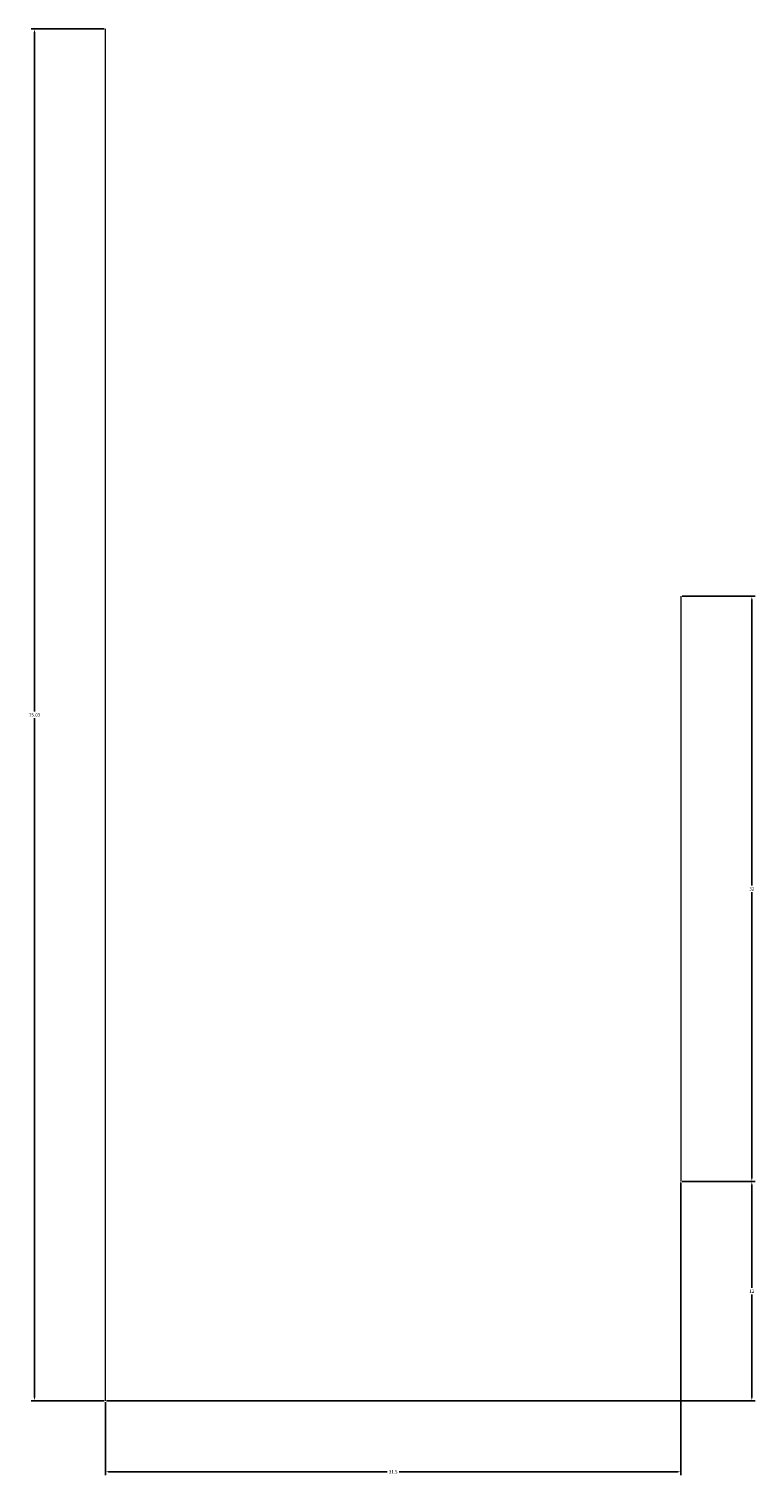
# Model space of a CAD drawing. Units: millimetres. Extents: x 554.6 to 594.4, y 996.2 to 1075.2.
import ezdxf

# ---------------------------------------------------------------- set-up
doc = ezdxf.new("R2010")
doc.units = ezdxf.units.MM
doc.layers.add('M-CONS', color=7, linetype='Continuous', lineweight=13)
doc.layers.add('M-DIMS', color=2, linetype='Continuous', lineweight=18)
doc.styles.get("Standard").update_dxf_attribs({"font": 'arial.ttf'})
doc.dimstyles.get("Standard").update_dxf_attribs({"dimtxt": 0.18, "dimasz": 0.18, "dimexe": 0.18, "dimexo": 0.0625, "dimgap": 0.09, "dimtad": 0, "dimtih": 1, "dimtoh": 1, "dimdec": 4, "dimzin": 0, "dimdsep": 46, "dimtxsty": 'Standard', "dimcen": 0.09, "dimadec": 0, "dimazin": 0, "dimtfac": 1, "dimtdec": 4, "dimtofl": 0, "dimtmove": 0, "dimatfit": 3, "dimfxl": 1, "dimtolj": 1, "dimtzin": 0, "dimarcsym": 0})

# ---------------------------------------------------------------- blocks, each defined once
blk = doc.blocks.new('*D1')
at = {"layer": 'Defpoints', "color": 0, "transparency": 16777216}
for p in [(554.956, 1075.245), (558.831, 1075.245), (558.831, 1000.216)]:
    blk.add_point(p, dxfattribs=at)
at = {"layer": 'M-DIMS', "color": 0, "lineweight": -2, "transparency": 16777216}
for p, q in [((558.768, 1075.245), (554.776, 1075.245)), ((554.956, 1075.065), (554.956, 1037.912)), ((554.956, 1000.396), (554.956, 1037.549)), ((558.768, 1000.216), (554.776, 1000.216))]:
    blk.add_line(p, q, dxfattribs=at)
at = {"layer": 'M-DIMS', "color": 0, "transparency": 16777216}
for points in [[(554.926, 1075.065), (554.986, 1075.065), (554.956, 1075.245)], [(554.926, 1000.396), (554.986, 1000.396), (554.956, 1000.216)]]:
    blk.add_solid(points, dxfattribs=at)
at = {"layer": 'M-DIMS', "color": 0, "transparency": 16777216, "insert": (554.956, 1037.73), "char_height": 0.18, "attachment_point": 5}
blk.add_mtext('\\A1;75.03', dxfattribs=at)
blk = doc.blocks.new('*D2')
at = {"layer": 'Defpoints', "color": 0, "transparency": 16777216}
for p in [(590.331, 1012.216), (558.831, 1000.216), (590.331, 996.341)]:
    blk.add_point(p, dxfattribs=at)
at = {"layer": 'M-DIMS', "color": 0, "lineweight": -2, "transparency": 16777216}
for p, q in [((590.331, 1012.153), (590.331, 996.161)), ((558.831, 1000.153), (558.831, 996.161)), ((559.011, 996.341), (574.256, 996.341)), ((590.151, 996.341), (574.905, 996.341))]:
    blk.add_line(p, q, dxfattribs=at)
at = {"layer": 'M-DIMS', "color": 0, "transparency": 16777216}
for points in [[(559.011, 996.371), (559.011, 996.311), (558.831, 996.341)], [(590.151, 996.371), (590.151, 996.311), (590.331, 996.341)]]:
    blk.add_solid(points, dxfattribs=at)
at = {"layer": 'M-DIMS', "color": 0, "transparency": 16777216, "insert": (574.581, 996.341), "char_height": 0.18, "attachment_point": 5}
blk.add_mtext('\\A1;31.5', dxfattribs=at)
blk = doc.blocks.new('*D3')
at = {"layer": 'Defpoints', "color": 0, "transparency": 16777216}
for p in [(590.331, 1044.216), (594.206, 1044.216), (590.331, 1012.216)]:
    blk.add_point(p, dxfattribs=at)
at = {"layer": 'M-DIMS', "color": 0, "lineweight": -2, "transparency": 16777216}
for p, q in [((590.393, 1044.216), (594.386, 1044.216)), ((594.206, 1044.036), (594.206, 1028.398)), ((594.206, 1012.396), (594.206, 1028.034)), ((590.393, 1012.216), (594.386, 1012.216))]:
    blk.add_line(p, q, dxfattribs=at)
at = {"layer": 'M-DIMS', "color": 0, "transparency": 16777216}
for points in [[(594.176, 1044.036), (594.236, 1044.036), (594.206, 1044.216)], [(594.176, 1012.396), (594.236, 1012.396), (594.206, 1012.216)]]:
    blk.add_solid(points, dxfattribs=at)
at = {"layer": 'M-DIMS', "color": 0, "transparency": 16777216, "insert": (594.206, 1028.216), "char_height": 0.18, "attachment_point": 5}
blk.add_mtext('\\A1;32', dxfattribs=at)
blk = doc.blocks.new('*D4')
at = {"layer": 'Defpoints', "color": 0, "transparency": 16777216}
for p in [(590.331, 1012.216), (594.206, 1012.216), (558.831, 1000.216)]:
    blk.add_point(p, dxfattribs=at)
at = {"layer": 'M-DIMS', "color": 0, "lineweight": -2, "transparency": 16777216}
for p, q in [((590.393, 1012.216), (594.386, 1012.216)), ((594.206, 1012.036), (594.206, 1006.396)), ((594.206, 1000.396), (594.206, 1006.035)), ((558.893, 1000.216), (594.386, 1000.216))]:
    blk.add_line(p, q, dxfattribs=at)
at = {"layer": 'M-DIMS', "color": 0, "transparency": 16777216}
for points in [[(594.176, 1012.036), (594.236, 1012.036), (594.206, 1012.216)], [(594.176, 1000.396), (594.236, 1000.396), (594.206, 1000.216)]]:
    blk.add_solid(points, dxfattribs=at)
at = {"layer": 'M-DIMS', "color": 0, "transparency": 16777216, "insert": (594.206, 1006.216), "char_height": 0.18, "attachment_point": 5}
blk.add_mtext('\\A1;12', dxfattribs=at)

msp = doc.modelspace()

# ---------------------------------------------------------------- linework, layer by layer
at = {"layer": 'M-CONS'}
for p, q in [((558.831, 1056.216, 18), (558.831, 1075.245, 38)), ((558.831, 1000.216, 18), (558.831, 1056.216, 63)), ((590.331, 1044.216), (590.331, 1044.216, 6)), ((590.331, 1044.216, 6), (590.331, 1012.216, 6)), ((590.331, 1012.216, 6), (590.331, 1012.216))]:
    msp.add_line(p, q, dxfattribs=at)

# ---------------------------------------------------------------- dimensions: what is measured, and where the dimension line sits
at = {"layer": 'M-DIMS'}
for base, p1, p2, override, picture, middle in [((554.956, 1075.245), (558.831, 1000.216), (558.831, 1075.245), {"dimdec": 2, "dimlfac": 1, "dimrnd": 0, "dimzin": 0, "dimdsep": 46, "dimlunit": 2}, '*D1', (554.956, 1037.73)), ((594.206, 1044.216), (590.331, 1012.216), (590.331, 1044.216), {"dimdec": 0, "dimlfac": 1, "dimrnd": 0, "dimzin": 0, "dimdsep": 46, "dimlunit": 2}, '*D3', (594.206, 1028.216)), ((594.206, 1012.216), (558.831, 1000.216), (590.331, 1012.216), {"dimdec": 0, "dimlfac": 1, "dimrnd": 0, "dimzin": 0, "dimdsep": 46, "dimlunit": 2}, '*D4', (594.206, 1006.216))]:
    dim = msp.add_linear_dim(base=base, p1=p1, p2=p2, angle=90, dimstyle='Standard', override=override, dxfattribs=at)
    dim.commit()
    dim.dimension.update_dxf_attribs({"geometry": picture, "text_midpoint": middle})
dim = msp.add_linear_dim(base=(590.331, 996.341), p1=(558.831, 1000.216), p2=(590.331, 1012.216), dimstyle='Standard', override={"dimdec": 1, "dimlfac": 1, "dimrnd": 0, "dimzin": 0, "dimdsep": 46, "dimlunit": 2}, dxfattribs=at)
dim.commit()
dim.dimension.update_dxf_attribs({"geometry": '*D2', "text_midpoint": (574.581, 996.341)})

doc.saveas('drawing.dxf')
